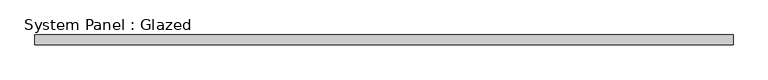
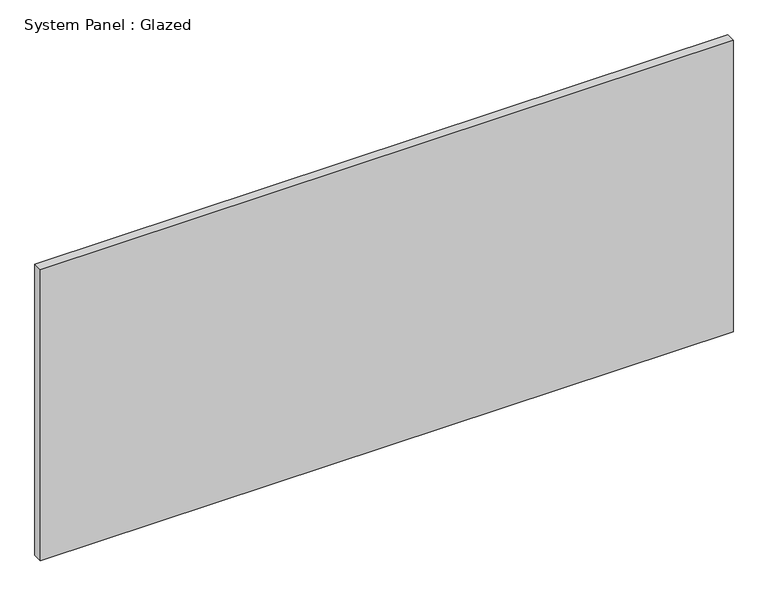
"""IFC4 building model written with IfcOpenShell, lengths in millimetres: plate geometry, System Panel : Glazed."""

from ifc_helpers import new_model, si_unit, origin, origin_with_axes, place, context, project, spatial, polyline, outline, extrude, source, transform, mapped, element, save


def system_panel_glazed_68ef09be(model_context):
    return source(origin(), model_context, "Body", "SweptSolid", [
        extrude(outline(polyline([(914.4, 19.05), (-914.4, 19.05), (-914.4, 44.45), (914.4, 44.45), (914.4, 19.05)])), origin_with_axes(), (0.0, 0.0, 1.0), 812.8),
    ])


if __name__ == "__main__":
    model = new_model("IFC4")
    model_context = context("Model", 3, world=origin())
    ifc_project = project(units=[si_unit("LENGTHUNIT", "METRE", prefix="MILLI")], contexts=[model_context])
    site = spatial("IfcSite", under=ifc_project)
    building = spatial("IfcBuilding", under=site)
    placement = place(None, origin())
    system_panel_glazed_shape = system_panel_glazed_68ef09be(model_context)
    element("IfcPlate", 1, ObjectType="System Panel : Glazed", at=placement, inside=building, context=model_context, shape_type="MappedRepresentation", body=[
        mapped(system_panel_glazed_shape, transform((0.0, 0.0, 0.0), x_axis=(1.0, 0.0, 0.0), y_axis=(0.0, 1.0, 0.0), z_axis=(0.0, 0.0, 1.0))),
    ])
    save(model, "model.ifc")

# Revit data of these elements
# Type "System Panel : Glazed"
#   Construction Type Id = "GSP4R"
#   Analytic Construction = "1/8 in Pilkington single glazing"
#   Visual Light Transmittance = 0.9
#   Solar Heat Gain Coefficient = 0.86
#   Heat Transfer Coefficient (U) = 1.18115 BTU/(h·ft²·°F)
# Element 1 (IfcPlate, "System Panel : Glazed")
#   Materials on its faces: "Glass"
# Materials
#   "Glass": class "Glass", colour RGB 0 128 192, transparency 0.75, Description = "Soda Lime Glass", Cost = 0
